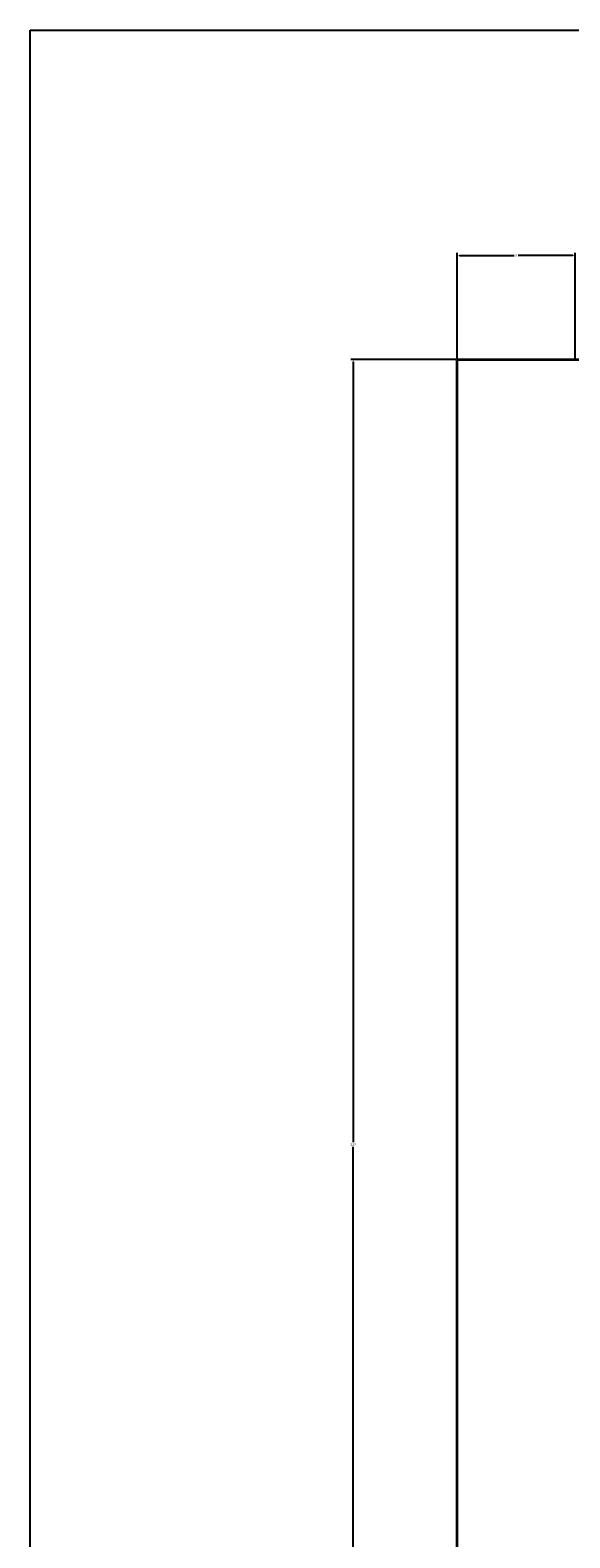
# Model space of a CAD drawing. Units: inches. Extents: x 4508 to 4723, y 847 to 1020.
# Tile 8 of 32: x 4508 to 4550, y 905 to 1020. Entities that reach past the tile are written whole.
import ezdxf

# ---------------------------------------------------------------- set-up
doc = ezdxf.new("R2010")
doc.units = ezdxf.units.IN
for name, color, linetype, lineweight in [('A-ANNO-DIMS', 2, 'Continuous', 18), ('A-ANNO-TTLB', 7, 'Continuous', 25), ('A-WALL', 7, 'Continuous', 35)]:
    doc.layers.add(name, color=color, linetype=linetype, lineweight=lineweight)
doc.styles.get("Standard").update_dxf_attribs({"font": 'arial.ttf'})
doc.dimstyles.get("Standard").update_dxf_attribs({"dimtxt": 0.18, "dimasz": 0.18, "dimexe": 0.18, "dimexo": 0.0625, "dimgap": 0.09, "dimtad": 0, "dimtih": 1, "dimtoh": 1, "dimdec": 4, "dimzin": 0, "dimdsep": 46, "dimtxsty": 'Standard', "dimcen": 0.09, "dimadec": 0, "dimazin": 0, "dimtfac": 1, "dimtdec": 4, "dimtofl": 0, "dimtmove": 0, "dimatfit": 3, "dimfxl": 1, "dimtolj": 1, "dimtzin": 0, "dimarcsym": 0})

# ---------------------------------------------------------------- blocks, each defined once
blk = doc.blocks.new('*D3')
at = {"layer": 'A-ANNO-DIMS', "color": 0, "lineweight": -2, "transparency": 16777216}
for p, q in [((4540.93, 994.75), (4532.86, 994.75)), ((4533.04, 994.57), (4533.04, 934.93)), ((4533.04, 874.93), (4533.04, 934.56)), ((4540.93, 874.75), (4532.86, 874.75))]:
    blk.add_line(p, q, dxfattribs=at)
at = {"layer": 'A-ANNO-DIMS', "color": 0, "lineweight": 9, "transparency": 16777216}
for points in [[(4533.01, 994.57), (4533.07, 994.57), (4533.04, 994.75)], [(4533.01, 874.93), (4533.07, 874.93), (4533.04, 874.75)]]:
    blk.add_solid(points, dxfattribs=at)
at = {"layer": 'Defpoints', "color": 0, "lineweight": 9, "transparency": 16777216}
for p in [(4533.04, 994.75), (4540.99, 994.75), (4540.99, 874.75)]:
    blk.add_point(p, dxfattribs=at)
at = {"layer": 'A-ANNO-DIMS', "color": 0, "transparency": 16777216, "insert": (4533.04, 934.75), "char_height": 0.18, "attachment_point": 5}
blk.add_mtext('\\A1;120', dxfattribs=at)
blk = doc.blocks.new('*D4')
at = {"layer": 'A-ANNO-DIMS', "color": 0, "lineweight": -2, "transparency": 16777216}
for p, q in [((4540.99, 994.81), (4540.99, 1002.88)), ((4541.17, 1002.7), (4545.34, 1002.7)), ((4549.81, 1002.7), (4545.64, 1002.7)), ((4549.99, 994.81), (4549.99, 1002.88))]:
    blk.add_line(p, q, dxfattribs=at)
at = {"layer": 'A-ANNO-DIMS', "color": 0, "lineweight": 9, "transparency": 16777216}
for points in [[(4541.17, 1002.73), (4541.17, 1002.67), (4540.99, 1002.7)], [(4549.81, 1002.73), (4549.81, 1002.67), (4549.99, 1002.7)]]:
    blk.add_solid(points, dxfattribs=at)
at = {"layer": 'Defpoints', "color": 0, "lineweight": 9, "transparency": 16777216}
for p in [(4549.99, 1002.7), (4540.99, 994.75), (4549.99, 994.75)]:
    blk.add_point(p, dxfattribs=at)
at = {"layer": 'A-ANNO-DIMS', "color": 0, "transparency": 16777216, "insert": (4545.49, 1002.7), "char_height": 0.18, "attachment_point": 5}
blk.add_mtext('\\A1;9', dxfattribs=at)

msp = doc.modelspace()

# ---------------------------------------------------------------- linework, layer by layer
at = {"layer": 'A-ANNO-TTLB'}
msp.add_lwpolyline([(4508.3867, 1019.9118), (4722.9774, 1019.9118), (4722.9774, 846.9535), (4508.3867, 846.9535)], close=True, dxfattribs=at)
at = {"layer": 'A-WALL'}
for p, q in [((4540.9938, 994.7469), (4693.9938, 994.7469)), ((4540.9938, 874.7469), (4540.9938, 994.7469))]:
    msp.add_line(p, q, dxfattribs=at)

# ---------------------------------------------------------------- dimensions: what is measured, and where the dimension line sits
at = {"layer": 'A-ANNO-DIMS'}
dim = msp.add_linear_dim(base=(4549.9938, 1002.6969), p1=(4540.9938, 994.7469), p2=(4549.9938, 994.7469), dimstyle='Standard', override={"dimdec": 0, "dimlfac": 1, "dimrnd": 0, "dimzin": 0, "dimdsep": 46, "dimlunit": 2}, dxfattribs=at)
dim.commit()
dim.dimension.update_dxf_attribs({"geometry": '*D4', "text_midpoint": (4545.4938, 1002.6969)})
dim = msp.add_linear_dim(base=(4533.0438, 994.7469), p1=(4540.9938, 874.7469), p2=(4540.9938, 994.7469), angle=90, dimstyle='Standard', override={"dimdec": 0, "dimlfac": 1, "dimrnd": 0, "dimzin": 0, "dimdsep": 46, "dimlunit": 2}, dxfattribs=at)
dim.commit()
dim.dimension.update_dxf_attribs({"geometry": '*D3', "text_midpoint": (4533.0438, 934.7469)})

doc.saveas('drawing.dxf')
